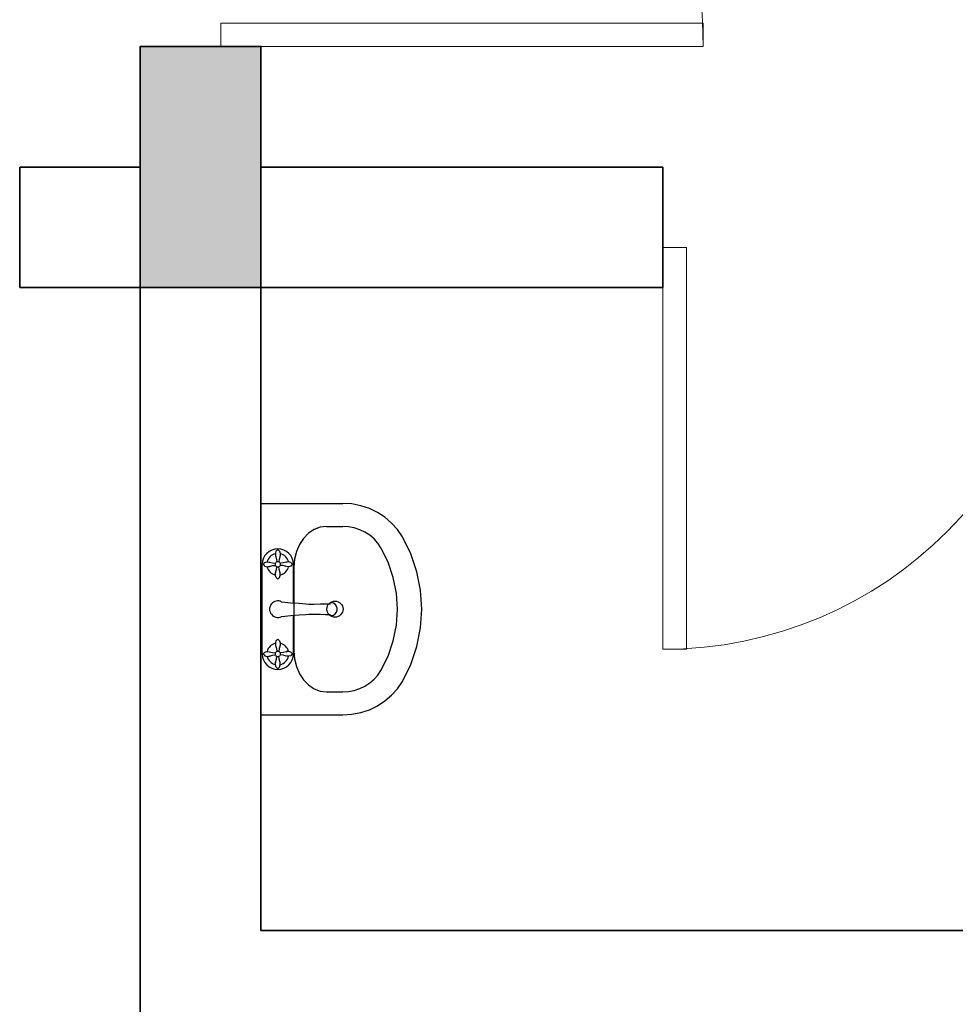
# Model space of a CAD drawing. Units: inches. Extents: x 3321 to 5237, y 11 to 1752.
# Tile 9 of 43: x 3654 to 3724, y 1372 to 1445. Entities that reach past the tile are written whole.
import ezdxf

# ---------------------------------------------------------------- set-up
doc = ezdxf.new("R2010")
doc.units = ezdxf.units.IN
for name, color, linetype, lineweight in [('A-ANNO-DIMS', 2, 'Continuous', 18), ('A-COLS', 1, 'Continuous', 35), ('A-DOOR', 4, 'Continuous', 18), ('A-WALL', 7, 'Continuous', 35), ('Сантехника', 7, 'Continuous', 18)]:
    doc.layers.add(name, color=color, linetype=linetype, lineweight=lineweight)
doc.layers.add('SANTEH', color=7, linetype='Continuous')
doc.styles.get("Standard").update_dxf_attribs({"font": 'arial.ttf'})
doc.dimstyles.new('ISO-25', dxfattribs={"dimtxt": 9, "dimasz": 2.5, "dimexe": 1.25, "dimexo": 0.625, "dimtad": 1, "dimdec": 1, "dimlunit": 3, "dimtxsty": 'Standard', "dimcen": 2.5, "dimclrd": 4, "dimclre": 4, "dimclrt": 256, "dimadec": 0, "dimazin": 0, "dimtfac": 1, "dimtdec": 1, "dimtmove": 0, "dimatfit": 3, "dimfxl": 1, "dimarcsym": 0})

# ---------------------------------------------------------------- blocks, each defined once
blk = doc.blocks.new('*U4')
for p, q in [((0, 0), (0, -6)), ((-36, 0), (-36, -6))]:
    blk.add_line(p, q)
blk.add_lwpolyline([(0, 0), (0, 36), (-1.75, 36), (-1.75, 0)], close=True)
blk.add_arc((0, 0), 36, 90, 180)
blk = doc.blocks.new('*U5')
for p, q in [((0, 0), (0, -6)), ((-30, 0), (-30, -6))]:
    blk.add_line(p, q)
blk.add_lwpolyline([(0, 0), (0, 30), (-1.75, 30), (-1.75, 0)], close=True)
blk.add_arc((0, 0), 30, 90, 180)
blk = doc.blocks.new('Basin 01_71')
at = {"layer": 'SANTEH'}
for p, q in [((0, 350), (0, 171.8)), ((460, 350), (0, 350)), ((130.2, 343.2), (128.5, 341.7)), ((130.2, 343.2), (128.5, 341.7)), ((130.2, 343.2), (128.5, 341.7)), ((130.2, 343.2), (128.5, 341.7)), ((130.2, 343.2), (128.5, 341.7)), ((130.2, 343.2), (128.5, 341.7)), ((132.5, 345.3), (130.2, 343.2)), ((132.5, 345.3), (130.2, 343.2)), ((132.5, 345.3), (130.2, 343.2)), ((132.5, 345.3), (130.2, 343.2)), ((132.5, 345.3), (130.2, 343.2)), ((132.5, 345.3), (130.2, 343.2)), ((132.5, 346.9), (327.5, 346.9)), ((132.5, 345.3), (134.7, 343.2)), ((132.5, 345.3), (134.7, 343.2)), ((132.5, 345.3), (134.7, 343.2)), ((132.5, 345.3), (134.7, 343.2)), ((132.5, 345.3), (134.7, 343.2)), ((132.5, 345.3), (134.7, 343.2)), ((134.7, 343.2), (136.4, 341.7)), ((134.7, 343.2), (136.4, 341.7)), ((134.7, 343.2), (136.4, 341.7)), ((134.7, 343.2), (136.4, 341.7)), ((134.7, 343.2), (136.4, 341.7)), ((134.7, 343.2), (136.4, 341.7)), ((325.2, 343.2), (323.5, 341.7)), ((325.2, 343.2), (323.5, 341.7)), ((325.2, 343.2), (323.5, 341.7)), ((325.2, 343.2), (323.5, 341.7)), ((325.2, 343.2), (323.5, 341.7)), ((325.2, 343.2), (323.5, 341.7)), ((327.5, 345.3), (325.2, 343.2)), ((327.5, 345.3), (325.2, 343.2)), ((327.5, 345.3), (325.2, 343.2)), ((327.5, 345.3), (325.2, 343.2)), ((327.5, 345.3), (325.2, 343.2)), ((327.5, 345.3), (325.2, 343.2)), ((327.5, 345.3), (329.7, 343.2)), ((327.5, 345.3), (329.7, 343.2)), ((327.5, 345.3), (329.7, 343.2)), ((327.5, 345.3), (329.7, 343.2)), ((327.5, 345.3), (329.7, 343.2)), ((327.5, 345.3), (329.7, 343.2)), ((329.7, 343.2), (331.4, 341.7)), ((329.7, 343.2), (331.4, 341.7)), ((329.7, 343.2), (331.4, 341.7)), ((329.7, 343.2), (331.4, 341.7)), ((329.7, 343.2), (331.4, 341.7)), ((329.7, 343.2), (331.4, 341.7)), ((460, 350), (460, 171.8)), ((128.5, 341.7), (127.2, 337.2)), ((128.5, 341.7), (127.2, 337.2)), ((128.5, 341.7), (127.2, 337.2)), ((128.5, 341.7), (127.2, 337.2)), ((128.5, 341.7), (127.2, 337.2)), ((128.5, 341.7), (127.2, 337.2)), ((127.2, 337.2), (127.5, 332.3)), ((127.2, 337.2), (127.5, 332.3)), ((127.2, 337.2), (127.5, 332.3)), ((127.2, 337.2), (127.5, 332.3)), ((127.2, 337.2), (127.5, 332.3)), ((127.2, 337.2), (127.5, 332.3)), ((127.5, 332.3), (128.4, 332)), ((127.5, 332.3), (128.4, 332)), ((127.5, 332.3), (128.4, 332)), ((127.5, 332.3), (128.4, 332)), ((127.5, 332.3), (128.4, 332)), ((127.5, 332.3), (128.4, 332)), ((128.4, 332), (127.6, 331.5)), ((128.4, 332), (127.6, 331.5)), ((128.4, 332), (127.6, 331.5)), ((128.4, 332), (127.6, 331.5)), ((128.4, 332), (127.6, 331.5)), ((128.4, 332), (127.6, 331.5)), ((127.6, 331.5), (129.6, 324.7)), ((127.6, 331.5), (129.6, 324.7)), ((127.6, 331.5), (129.6, 324.7)), ((127.6, 331.5), (129.6, 324.7)), ((127.6, 331.5), (129.6, 324.7)), ((127.6, 331.5), (129.6, 324.7)), ((129.6, 324.7), (130.2, 318.4)), ((129.6, 324.7), (130.2, 318.4)), ((129.6, 324.7), (130.2, 318.4)), ((129.6, 324.7), (130.2, 318.4)), ((129.6, 324.7), (130.2, 318.4)), ((129.6, 324.7), (130.2, 318.4)), ((135.4, 324.7), (134.8, 318.4)), ((135.4, 324.7), (134.8, 318.4)), ((135.4, 324.7), (134.8, 318.4)), ((135.4, 324.7), (134.8, 318.4)), ((135.4, 324.7), (134.8, 318.4)), ((135.4, 324.7), (134.8, 318.4)), ((137.4, 331.5), (135.4, 324.7)), ((137.4, 331.5), (135.4, 324.7)), ((137.4, 331.5), (135.4, 324.7)), ((137.4, 331.5), (135.4, 324.7)), ((137.4, 331.5), (135.4, 324.7)), ((137.4, 331.5), (135.4, 324.7)), ((136.4, 341.7), (137.7, 337.2)), ((136.4, 341.7), (137.7, 337.2)), ((136.4, 341.7), (137.7, 337.2)), ((136.4, 341.7), (137.7, 337.2)), ((136.4, 341.7), (137.7, 337.2)), ((136.4, 341.7), (137.7, 337.2)), ((137.4, 332.3), (136.6, 332)), ((137.4, 332.3), (136.6, 332)), ((137.4, 332.3), (136.6, 332)), ((137.4, 332.3), (136.6, 332)), ((137.4, 332.3), (136.6, 332)), ((137.4, 332.3), (136.6, 332)), ((136.6, 332), (137.4, 331.5)), ((136.6, 332), (137.4, 331.5)), ((136.6, 332), (137.4, 331.5)), ((136.6, 332), (137.4, 331.5)), ((136.6, 332), (137.4, 331.5)), ((136.6, 332), (137.4, 331.5)), ((137.7, 337.2), (137.4, 332.3)), ((137.7, 337.2), (137.4, 332.3)), ((137.7, 337.2), (137.4, 332.3)), ((137.7, 337.2), (137.4, 332.3)), ((137.7, 337.2), (137.4, 332.3)), ((137.7, 337.2), (137.4, 332.3)), ((323.5, 341.7), (322.2, 337.2)), ((323.5, 341.7), (322.2, 337.2)), ((323.5, 341.7), (322.2, 337.2)), ((323.5, 341.7), (322.2, 337.2)), ((323.5, 341.7), (322.2, 337.2)), ((323.5, 341.7), (322.2, 337.2)), ((322.2, 337.2), (322.5, 332.3)), ((322.2, 337.2), (322.5, 332.3)), ((322.2, 337.2), (322.5, 332.3)), ((322.2, 337.2), (322.5, 332.3)), ((322.2, 337.2), (322.5, 332.3)), ((322.2, 337.2), (322.5, 332.3)), ((322.5, 332.3), (323.4, 332)), ((322.5, 332.3), (323.4, 332)), ((322.5, 332.3), (323.4, 332)), ((322.5, 332.3), (323.4, 332)), ((322.5, 332.3), (323.4, 332)), ((322.5, 332.3), (323.4, 332)), ((323.4, 332), (322.6, 331.5)), ((323.4, 332), (322.6, 331.5)), ((323.4, 332), (322.6, 331.5)), ((323.4, 332), (322.6, 331.5)), ((323.4, 332), (322.6, 331.5)), ((323.4, 332), (322.6, 331.5)), ((322.6, 331.5), (324.6, 324.7)), ((322.6, 331.5), (324.6, 324.7)), ((322.6, 331.5), (324.6, 324.7)), ((322.6, 331.5), (324.6, 324.7)), ((322.6, 331.5), (324.6, 324.7)), ((322.6, 331.5), (324.6, 324.7)), ((324.6, 324.7), (325.2, 318.4)), ((324.6, 324.7), (325.2, 318.4)), ((324.6, 324.7), (325.2, 318.4)), ((324.6, 324.7), (325.2, 318.4)), ((324.6, 324.7), (325.2, 318.4)), ((324.6, 324.7), (325.2, 318.4)), ((330.4, 324.7), (329.8, 318.4)), ((330.4, 324.7), (329.8, 318.4)), ((330.4, 324.7), (329.8, 318.4)), ((330.4, 324.7), (329.8, 318.4)), ((330.4, 324.7), (329.8, 318.4)), ((330.4, 324.7), (329.8, 318.4)), ((332.4, 331.5), (330.4, 324.7)), ((332.4, 331.5), (330.4, 324.7)), ((332.4, 331.5), (330.4, 324.7)), ((332.4, 331.5), (330.4, 324.7)), ((332.4, 331.5), (330.4, 324.7)), ((332.4, 331.5), (330.4, 324.7)), ((331.4, 341.7), (332.7, 337.2)), ((331.4, 341.7), (332.7, 337.2)), ((331.4, 341.7), (332.7, 337.2)), ((331.4, 341.7), (332.7, 337.2)), ((331.4, 341.7), (332.7, 337.2)), ((331.4, 341.7), (332.7, 337.2)), ((332.4, 332.3), (331.6, 332)), ((332.4, 332.3), (331.6, 332)), ((332.4, 332.3), (331.6, 332)), ((332.4, 332.3), (331.6, 332)), ((332.4, 332.3), (331.6, 332)), ((332.4, 332.3), (331.6, 332)), ((331.6, 332), (332.4, 331.5)), ((331.6, 332), (332.4, 331.5)), ((331.6, 332), (332.4, 331.5)), ((331.6, 332), (332.4, 331.5)), ((331.6, 332), (332.4, 331.5)), ((331.6, 332), (332.4, 331.5)), ((332.7, 337.2), (332.4, 332.3)), ((332.7, 337.2), (332.4, 332.3)), ((332.7, 337.2), (332.4, 332.3)), ((332.7, 337.2), (332.4, 332.3)), ((332.7, 337.2), (332.4, 332.3)), ((332.7, 337.2), (332.4, 332.3)), ((100.4, 313.2), (102.5, 315.4)), ((100.4, 313.2), (102.5, 315.4)), ((100.4, 313.2), (102.5, 315.4)), ((100.4, 313.2), (102.5, 315.4)), ((100.4, 313.2), (102.5, 315.4)), ((100.4, 313.2), (102.5, 315.4)), ((100.4, 313.2), (102.5, 310.9)), ((100.4, 313.2), (102.5, 310.9)), ((100.4, 313.2), (102.5, 310.9)), ((100.4, 313.2), (102.5, 310.9)), ((100.4, 313.2), (102.5, 310.9)), ((100.4, 313.2), (102.5, 310.9)), ((102.5, 315.4), (104, 317.1)), ((102.5, 315.4), (104, 317.1)), ((102.5, 315.4), (104, 317.1)), ((102.5, 315.4), (104, 317.1)), ((102.5, 315.4), (104, 317.1)), ((102.5, 315.4), (104, 317.1)), ((102.5, 310.9), (104, 309.2)), ((102.5, 310.9), (104, 309.2)), ((102.5, 310.9), (104, 309.2)), ((102.5, 310.9), (104, 309.2)), ((102.5, 310.9), (104, 309.2)), ((102.5, 310.9), (104, 309.2)), ((104, 317.1), (108.5, 318.4)), ((104, 317.1), (108.5, 318.4)), ((104, 317.1), (108.5, 318.4)), ((104, 317.1), (108.5, 318.4)), ((104, 317.1), (108.5, 318.4)), ((104, 317.1), (108.5, 318.4)), ((104, 309.2), (108.5, 307.9)), ((104, 309.2), (108.5, 307.9)), ((104, 309.2), (108.5, 307.9)), ((104, 309.2), (108.5, 307.9)), ((104, 309.2), (108.5, 307.9)), ((104, 309.2), (108.5, 307.9)), ((108.5, 318.4), (113.4, 318.1)), ((108.5, 318.4), (113.4, 318.1)), ((108.5, 318.4), (113.4, 318.1)), ((108.5, 318.4), (113.4, 318.1)), ((108.5, 318.4), (113.4, 318.1)), ((108.5, 318.4), (113.4, 318.1)), ((108.5, 307.9), (113.4, 308.2)), ((108.5, 307.9), (113.4, 308.2)), ((108.5, 307.9), (113.4, 308.2)), ((108.5, 307.9), (113.4, 308.2)), ((108.5, 307.9), (113.4, 308.2)), ((108.5, 307.9), (113.4, 308.2)), ((113.4, 318.1), (113.7, 317.3)), ((113.4, 318.1), (113.7, 317.3)), ((113.4, 318.1), (113.7, 317.3)), ((113.4, 318.1), (113.7, 317.3)), ((113.4, 318.1), (113.7, 317.3)), ((113.4, 318.1), (113.7, 317.3)), ((113.4, 308.2), (113.7, 309.1)), ((113.4, 308.2), (113.7, 309.1)), ((113.4, 308.2), (113.7, 309.1)), ((113.4, 308.2), (113.7, 309.1)), ((113.4, 308.2), (113.7, 309.1)), ((113.4, 308.2), (113.7, 309.1)), ((113.7, 317.3), (114.2, 318.1)), ((113.7, 317.3), (114.2, 318.1)), ((113.7, 317.3), (114.2, 318.1)), ((113.7, 317.3), (114.2, 318.1)), ((113.7, 317.3), (114.2, 318.1)), ((113.7, 317.3), (114.2, 318.1)), ((113.7, 309.1), (114.2, 308.3)), ((113.7, 309.1), (114.2, 308.3)), ((113.7, 309.1), (114.2, 308.3)), ((113.7, 309.1), (114.2, 308.3)), ((113.7, 309.1), (114.2, 308.3)), ((113.7, 309.1), (114.2, 308.3)), ((114.2, 318.1), (121, 316.1)), ((114.2, 318.1), (121, 316.1)), ((114.2, 318.1), (121, 316.1)), ((114.2, 318.1), (121, 316.1)), ((114.2, 318.1), (121, 316.1)), ((114.2, 318.1), (121, 316.1)), ((114.2, 308.3), (121, 310.3)), ((114.2, 308.3), (121, 310.3)), ((114.2, 308.3), (121, 310.3)), ((114.2, 308.3), (121, 310.3)), ((114.2, 308.3), (121, 310.3)), ((114.2, 308.3), (121, 310.3)), ((121, 316.1), (127.3, 315.5)), ((121, 316.1), (127.3, 315.5)), ((121, 316.1), (127.3, 315.5)), ((121, 316.1), (127.3, 315.5)), ((121, 316.1), (127.3, 315.5)), ((121, 316.1), (127.3, 315.5)), ((121, 310.3), (127.3, 310.9)), ((121, 310.3), (127.3, 310.9)), ((121, 310.3), (127.3, 310.9)), ((121, 310.3), (127.3, 310.9)), ((121, 310.3), (127.3, 310.9)), ((121, 310.3), (127.3, 310.9)), ((127.1, 315.1), (126.8, 313.9)), ((127.1, 315.1), (126.8, 313.9)), ((127.1, 315.1), (126.8, 313.9)), ((127.1, 315.1), (126.8, 313.9)), ((127.1, 315.1), (126.8, 313.9)), ((127.1, 315.1), (126.8, 313.9)), ((126.8, 313.9), (126.8, 312.5)), ((126.8, 313.9), (126.8, 312.5)), ((126.8, 313.9), (126.8, 312.5)), ((126.8, 313.9), (126.8, 312.5)), ((126.8, 313.9), (126.8, 312.5)), ((126.8, 313.9), (126.8, 312.5)), ((126.8, 312.5), (127.1, 311.2)), ((126.8, 312.5), (127.1, 311.2)), ((126.8, 312.5), (127.1, 311.2)), ((126.8, 312.5), (127.1, 311.2)), ((126.8, 312.5), (127.1, 311.2)), ((126.8, 312.5), (127.1, 311.2)), ((127.7, 316.3), (127.1, 315.1)), ((127.7, 316.3), (127.1, 315.1)), ((127.7, 316.3), (127.1, 315.1)), ((127.7, 316.3), (127.1, 315.1)), ((127.7, 316.3), (127.1, 315.1)), ((127.7, 316.3), (127.1, 315.1)), ((127.1, 311.2), (127.7, 310.1)), ((127.1, 311.2), (127.7, 310.1)), ((127.1, 311.2), (127.7, 310.1)), ((127.1, 311.2), (127.7, 310.1)), ((127.1, 311.2), (127.7, 310.1)), ((127.1, 311.2), (127.7, 310.1)), ((127.6, 294.9), (129.6, 301.7)), ((127.6, 294.9), (129.6, 301.7)), ((127.6, 294.9), (129.6, 301.7)), ((127.6, 294.9), (129.6, 301.7)), ((127.6, 294.9), (129.6, 301.7)), ((127.6, 294.9), (129.6, 301.7)), ((128.6, 317.3), (127.7, 316.3)), ((128.6, 317.3), (127.7, 316.3)), ((128.6, 317.3), (127.7, 316.3)), ((128.6, 317.3), (127.7, 316.3)), ((128.6, 317.3), (127.7, 316.3)), ((128.6, 317.3), (127.7, 316.3)), ((127.7, 310.1), (128.6, 309.1)), ((127.7, 310.1), (128.6, 309.1)), ((127.7, 310.1), (128.6, 309.1)), ((127.7, 310.1), (128.6, 309.1)), ((127.7, 310.1), (128.6, 309.1)), ((127.7, 310.1), (128.6, 309.1)), ((129.7, 318.1), (128.6, 317.3)), ((129.7, 318.1), (128.6, 317.3)), ((129.7, 318.1), (128.6, 317.3)), ((129.7, 318.1), (128.6, 317.3)), ((129.7, 318.1), (128.6, 317.3)), ((129.7, 318.1), (128.6, 317.3)), ((128.6, 309.1), (129.7, 308.3)), ((128.6, 309.1), (129.7, 308.3)), ((128.6, 309.1), (129.7, 308.3)), ((128.6, 309.1), (129.7, 308.3)), ((128.6, 309.1), (129.7, 308.3)), ((128.6, 309.1), (129.7, 308.3)), ((129.6, 301.7), (130.2, 308)), ((129.6, 301.7), (130.2, 308)), ((129.6, 301.7), (130.2, 308)), ((129.6, 301.7), (130.2, 308)), ((129.6, 301.7), (130.2, 308)), ((129.6, 301.7), (130.2, 308)), ((130.9, 318.7), (129.7, 318.1)), ((130.9, 318.7), (129.7, 318.1)), ((130.9, 318.7), (129.7, 318.1)), ((130.9, 318.7), (129.7, 318.1)), ((130.9, 318.7), (129.7, 318.1)), ((130.9, 318.7), (129.7, 318.1)), ((129.7, 308.3), (130.9, 307.7)), ((129.7, 308.3), (130.9, 307.7)), ((129.7, 308.3), (130.9, 307.7)), ((129.7, 308.3), (130.9, 307.7)), ((129.7, 308.3), (130.9, 307.7)), ((129.7, 308.3), (130.9, 307.7)), ((132.2, 318.9), (130.9, 318.7)), ((132.2, 318.9), (130.9, 318.7)), ((132.2, 318.9), (130.9, 318.7)), ((132.2, 318.9), (130.9, 318.7)), ((132.2, 318.9), (130.9, 318.7)), ((132.2, 318.9), (130.9, 318.7)), ((130.9, 307.7), (132.2, 307.5)), ((130.9, 307.7), (132.2, 307.5)), ((130.9, 307.7), (132.2, 307.5)), ((130.9, 307.7), (132.2, 307.5)), ((130.9, 307.7), (132.2, 307.5)), ((130.9, 307.7), (132.2, 307.5)), ((133.5, 318.8), (132.2, 318.9)), ((133.5, 318.8), (132.2, 318.9)), ((133.5, 318.8), (132.2, 318.9)), ((133.5, 318.8), (132.2, 318.9)), ((133.5, 318.8), (132.2, 318.9)), ((133.5, 318.8), (132.2, 318.9)), ((132.2, 307.5), (133.5, 307.6)), ((132.2, 307.5), (133.5, 307.6)), ((132.2, 307.5), (133.5, 307.6)), ((132.2, 307.5), (133.5, 307.6)), ((132.2, 307.5), (133.5, 307.6)), ((132.2, 307.5), (133.5, 307.6)), ((134.8, 318.4), (133.5, 318.8)), ((134.8, 318.4), (133.5, 318.8)), ((134.8, 318.4), (133.5, 318.8)), ((134.8, 318.4), (133.5, 318.8)), ((134.8, 318.4), (133.5, 318.8)), ((134.8, 318.4), (133.5, 318.8)), ((133.5, 307.6), (134.8, 308)), ((133.5, 307.6), (134.8, 308)), ((133.5, 307.6), (134.8, 308)), ((133.5, 307.6), (134.8, 308)), ((133.5, 307.6), (134.8, 308)), ((133.5, 307.6), (134.8, 308)), ((135.9, 317.8), (134.8, 318.4)), ((135.9, 317.8), (134.8, 318.4)), ((135.9, 317.8), (134.8, 318.4)), ((135.9, 317.8), (134.8, 318.4)), ((135.9, 317.8), (134.8, 318.4)), ((135.9, 317.8), (134.8, 318.4)), ((134.8, 308), (135.9, 308.6)), ((134.8, 308), (135.9, 308.6)), ((134.8, 308), (135.9, 308.6)), ((134.8, 308), (135.9, 308.6)), ((134.8, 308), (135.9, 308.6)), ((134.8, 308), (135.9, 308.6)), ((135.4, 301.7), (134.8, 308)), ((135.4, 301.7), (134.8, 308)), ((135.4, 301.7), (134.8, 308)), ((135.4, 301.7), (134.8, 308)), ((135.4, 301.7), (134.8, 308)), ((135.4, 301.7), (134.8, 308)), ((137.4, 294.9), (135.4, 301.7)), ((137.4, 294.9), (135.4, 301.7)), ((137.4, 294.9), (135.4, 301.7)), ((137.4, 294.9), (135.4, 301.7)), ((137.4, 294.9), (135.4, 301.7)), ((137.4, 294.9), (135.4, 301.7)), ((136.9, 316.9), (135.9, 317.8)), ((136.9, 316.9), (135.9, 317.8)), ((136.9, 316.9), (135.9, 317.8)), ((136.9, 316.9), (135.9, 317.8)), ((136.9, 316.9), (135.9, 317.8)), ((136.9, 316.9), (135.9, 317.8)), ((135.9, 308.6), (136.9, 309.5)), ((135.9, 308.6), (136.9, 309.5)), ((135.9, 308.6), (136.9, 309.5)), ((135.9, 308.6), (136.9, 309.5)), ((135.9, 308.6), (136.9, 309.5)), ((135.9, 308.6), (136.9, 309.5)), ((137.6, 315.8), (136.9, 316.9)), ((137.6, 315.8), (136.9, 316.9)), ((137.6, 315.8), (136.9, 316.9)), ((137.6, 315.8), (136.9, 316.9)), ((137.6, 315.8), (136.9, 316.9)), ((137.6, 315.8), (136.9, 316.9)), ((136.9, 309.5), (137.6, 310.6)), ((136.9, 309.5), (137.6, 310.6)), ((136.9, 309.5), (137.6, 310.6)), ((136.9, 309.5), (137.6, 310.6)), ((136.9, 309.5), (137.6, 310.6)), ((136.9, 309.5), (137.6, 310.6)), ((138, 314.5), (137.6, 315.8)), ((138, 314.5), (137.6, 315.8)), ((138, 314.5), (137.6, 315.8)), ((138, 314.5), (137.6, 315.8)), ((138, 314.5), (137.6, 315.8)), ((138, 314.5), (137.6, 315.8)), ((137.6, 310.6), (138, 311.9)), ((137.6, 310.6), (138, 311.9)), ((137.6, 310.6), (138, 311.9)), ((137.6, 310.6), (138, 311.9)), ((137.6, 310.6), (138, 311.9)), ((137.6, 310.6), (138, 311.9)), ((144, 316.1), (137.7, 315.5)), ((144, 316.1), (137.7, 315.5)), ((144, 316.1), (137.7, 315.5)), ((144, 316.1), (137.7, 315.5)), ((144, 316.1), (137.7, 315.5)), ((144, 316.1), (137.7, 315.5)), ((144, 310.3), (137.7, 310.9)), ((144, 310.3), (137.7, 310.9)), ((144, 310.3), (137.7, 310.9)), ((144, 310.3), (137.7, 310.9)), ((144, 310.3), (137.7, 310.9)), ((144, 310.3), (137.7, 310.9)), ((138.2, 313.2), (138, 314.5)), ((138.2, 313.2), (138, 314.5)), ((138.2, 313.2), (138, 314.5)), ((138.2, 313.2), (138, 314.5)), ((138.2, 313.2), (138, 314.5)), ((138.2, 313.2), (138, 314.5)), ((138, 311.9), (138.2, 313.2)), ((138, 311.9), (138.2, 313.2)), ((138, 311.9), (138.2, 313.2)), ((138, 311.9), (138.2, 313.2)), ((138, 311.9), (138.2, 313.2)), ((138, 311.9), (138.2, 313.2)), ((150.8, 318.1), (144, 316.1)), ((150.8, 318.1), (144, 316.1)), ((150.8, 318.1), (144, 316.1)), ((150.8, 318.1), (144, 316.1)), ((150.8, 318.1), (144, 316.1)), ((150.8, 318.1), (144, 316.1)), ((150.8, 308.3), (144, 310.3)), ((150.8, 308.3), (144, 310.3)), ((150.8, 308.3), (144, 310.3)), ((150.8, 308.3), (144, 310.3)), ((150.8, 308.3), (144, 310.3)), ((150.8, 308.3), (144, 310.3)), ((151.3, 317.3), (150.8, 318.1)), ((151.3, 317.3), (150.8, 318.1)), ((151.3, 317.3), (150.8, 318.1)), ((151.3, 317.3), (150.8, 318.1)), ((151.3, 317.3), (150.8, 318.1)), ((151.3, 317.3), (150.8, 318.1)), ((151.3, 309.1), (150.8, 308.3)), ((151.3, 309.1), (150.8, 308.3)), ((151.3, 309.1), (150.8, 308.3)), ((151.3, 309.1), (150.8, 308.3)), ((151.3, 309.1), (150.8, 308.3)), ((151.3, 309.1), (150.8, 308.3)), ((151.6, 318.1), (151.3, 317.3)), ((151.6, 318.1), (151.3, 317.3)), ((151.6, 318.1), (151.3, 317.3)), ((151.6, 318.1), (151.3, 317.3)), ((151.6, 318.1), (151.3, 317.3)), ((151.6, 318.1), (151.3, 317.3)), ((151.6, 308.3), (151.3, 309.1)), ((151.6, 308.3), (151.3, 309.1)), ((151.6, 308.3), (151.3, 309.1)), ((151.6, 308.3), (151.3, 309.1)), ((151.6, 308.3), (151.3, 309.1)), ((151.6, 308.3), (151.3, 309.1)), ((156.5, 318.4), (151.6, 318.1)), ((156.5, 318.4), (151.6, 318.1)), ((156.5, 318.4), (151.6, 318.1)), ((156.5, 318.4), (151.6, 318.1)), ((156.5, 318.4), (151.6, 318.1)), ((156.5, 318.4), (151.6, 318.1)), ((156.5, 308), (151.6, 308.3)), ((156.5, 308), (151.6, 308.3)), ((156.5, 308), (151.6, 308.3)), ((156.5, 308), (151.6, 308.3)), ((156.5, 308), (151.6, 308.3)), ((156.5, 308), (151.6, 308.3)), ((161, 317.2), (156.5, 318.4)), ((161, 317.2), (156.5, 318.4)), ((161, 317.2), (156.5, 318.4)), ((161, 317.2), (156.5, 318.4)), ((161, 317.2), (156.5, 318.4)), ((161, 317.2), (156.5, 318.4)), ((161, 309.2), (156.5, 308)), ((161, 309.2), (156.5, 308)), ((161, 309.2), (156.5, 308)), ((161, 309.2), (156.5, 308)), ((161, 309.2), (156.5, 308)), ((161, 309.2), (156.5, 308)), ((162.5, 315.4), (161, 317.2)), ((162.5, 315.4), (161, 317.2)), ((162.5, 315.4), (161, 317.2)), ((162.5, 315.4), (161, 317.2)), ((162.5, 315.4), (161, 317.2)), ((162.5, 315.4), (161, 317.2)), ((162.5, 311), (161, 309.2)), ((162.5, 311), (161, 309.2)), ((162.5, 311), (161, 309.2)), ((162.5, 311), (161, 309.2)), ((162.5, 311), (161, 309.2)), ((162.5, 311), (161, 309.2)), ((164.6, 313.2), (162.5, 315.4)), ((164.6, 313.2), (162.5, 315.4)), ((164.6, 313.2), (162.5, 315.4)), ((164.6, 313.2), (162.5, 315.4)), ((164.6, 313.2), (162.5, 315.4)), ((164.6, 313.2), (162.5, 315.4)), ((164.6, 313.2), (162.5, 311)), ((164.6, 313.2), (162.5, 311)), ((164.6, 313.2), (162.5, 311)), ((164.6, 313.2), (162.5, 311)), ((164.6, 313.2), (162.5, 311)), ((164.6, 313.2), (162.5, 311)), ((213.9, 305.1), (215, 298)), ((246.1, 305.1), (245, 298)), ((295.4, 313.2), (297.5, 315.4)), ((295.4, 313.2), (297.5, 315.4)), ((295.4, 313.2), (297.5, 315.4)), ((295.4, 313.2), (297.5, 315.4)), ((295.4, 313.2), (297.5, 315.4)), ((295.4, 313.2), (297.5, 315.4)), ((295.4, 313.2), (297.5, 310.9)), ((295.4, 313.2), (297.5, 310.9)), ((295.4, 313.2), (297.5, 310.9)), ((295.4, 313.2), (297.5, 310.9)), ((295.4, 313.2), (297.5, 310.9)), ((295.4, 313.2), (297.5, 310.9)), ((297.5, 315.4), (299, 317.1)), ((297.5, 315.4), (299, 317.1)), ((297.5, 315.4), (299, 317.1)), ((297.5, 315.4), (299, 317.1)), ((297.5, 315.4), (299, 317.1)), ((297.5, 315.4), (299, 317.1)), ((297.5, 310.9), (299, 309.2)), ((297.5, 310.9), (299, 309.2)), ((297.5, 310.9), (299, 309.2)), ((297.5, 310.9), (299, 309.2)), ((297.5, 310.9), (299, 309.2)), ((297.5, 310.9), (299, 309.2)), ((299, 317.1), (303.5, 318.4)), ((299, 317.1), (303.5, 318.4)), ((299, 317.1), (303.5, 318.4)), ((299, 317.1), (303.5, 318.4)), ((299, 317.1), (303.5, 318.4)), ((299, 317.1), (303.5, 318.4)), ((299, 309.2), (303.5, 307.9)), ((299, 309.2), (303.5, 307.9)), ((299, 309.2), (303.5, 307.9)), ((299, 309.2), (303.5, 307.9)), ((299, 309.2), (303.5, 307.9)), ((299, 309.2), (303.5, 307.9)), ((303.5, 318.4), (308.4, 318.1)), ((303.5, 318.4), (308.4, 318.1)), ((303.5, 318.4), (308.4, 318.1)), ((303.5, 318.4), (308.4, 318.1)), ((303.5, 318.4), (308.4, 318.1)), ((303.5, 318.4), (308.4, 318.1)), ((303.5, 307.9), (308.4, 308.2)), ((303.5, 307.9), (308.4, 308.2)), ((303.5, 307.9), (308.4, 308.2)), ((303.5, 307.9), (308.4, 308.2)), ((303.5, 307.9), (308.4, 308.2)), ((303.5, 307.9), (308.4, 308.2)), ((308.4, 318.1), (308.7, 317.3)), ((308.4, 318.1), (308.7, 317.3)), ((308.4, 318.1), (308.7, 317.3)), ((308.4, 318.1), (308.7, 317.3)), ((308.4, 318.1), (308.7, 317.3)), ((308.4, 318.1), (308.7, 317.3)), ((308.4, 308.2), (308.7, 309.1)), ((308.4, 308.2), (308.7, 309.1)), ((308.4, 308.2), (308.7, 309.1)), ((308.4, 308.2), (308.7, 309.1)), ((308.4, 308.2), (308.7, 309.1)), ((308.4, 308.2), (308.7, 309.1)), ((308.7, 317.3), (309.2, 318.1)), ((308.7, 317.3), (309.2, 318.1)), ((308.7, 317.3), (309.2, 318.1)), ((308.7, 317.3), (309.2, 318.1)), ((308.7, 317.3), (309.2, 318.1)), ((308.7, 317.3), (309.2, 318.1)), ((308.7, 309.1), (309.2, 308.3)), ((308.7, 309.1), (309.2, 308.3)), ((308.7, 309.1), (309.2, 308.3)), ((308.7, 309.1), (309.2, 308.3)), ((308.7, 309.1), (309.2, 308.3)), ((308.7, 309.1), (309.2, 308.3)), ((309.2, 318.1), (316, 316.1)), ((309.2, 318.1), (316, 316.1)), ((309.2, 318.1), (316, 316.1)), ((309.2, 318.1), (316, 316.1)), ((309.2, 318.1), (316, 316.1)), ((309.2, 318.1), (316, 316.1)), ((309.2, 308.3), (316, 310.3)), ((309.2, 308.3), (316, 310.3)), ((309.2, 308.3), (316, 310.3)), ((309.2, 308.3), (316, 310.3)), ((309.2, 308.3), (316, 310.3)), ((309.2, 308.3), (316, 310.3)), ((316, 316.1), (322.3, 315.5)), ((316, 316.1), (322.3, 315.5)), ((316, 316.1), (322.3, 315.5)), ((316, 316.1), (322.3, 315.5)), ((316, 316.1), (322.3, 315.5)), ((316, 316.1), (322.3, 315.5)), ((316, 310.3), (322.3, 310.9)), ((316, 310.3), (322.3, 310.9)), ((316, 310.3), (322.3, 310.9)), ((316, 310.3), (322.3, 310.9)), ((316, 310.3), (322.3, 310.9)), ((316, 310.3), (322.3, 310.9)), ((322.1, 315.1), (321.8, 313.9)), ((322.1, 315.1), (321.8, 313.9)), ((322.1, 315.1), (321.8, 313.9)), ((322.1, 315.1), (321.8, 313.9)), ((322.1, 315.1), (321.8, 313.9)), ((322.1, 315.1), (321.8, 313.9)), ((321.8, 313.9), (321.8, 312.5)), ((321.8, 313.9), (321.8, 312.5)), ((321.8, 313.9), (321.8, 312.5)), ((321.8, 313.9), (321.8, 312.5)), ((321.8, 313.9), (321.8, 312.5)), ((321.8, 313.9), (321.8, 312.5)), ((321.8, 312.5), (322.1, 311.2)), ((321.8, 312.5), (322.1, 311.2)), ((321.8, 312.5), (322.1, 311.2)), ((321.8, 312.5), (322.1, 311.2)), ((321.8, 312.5), (322.1, 311.2)), ((321.8, 312.5), (322.1, 311.2)), ((322.7, 316.3), (322.1, 315.1)), ((322.7, 316.3), (322.1, 315.1)), ((322.7, 316.3), (322.1, 315.1)), ((322.7, 316.3), (322.1, 315.1)), ((322.7, 316.3), (322.1, 315.1)), ((322.7, 316.3), (322.1, 315.1)), ((322.1, 311.2), (322.7, 310.1)), ((322.1, 311.2), (322.7, 310.1)), ((322.1, 311.2), (322.7, 310.1)), ((322.1, 311.2), (322.7, 310.1)), ((322.1, 311.2), (322.7, 310.1)), ((322.1, 311.2), (322.7, 310.1)), ((322.6, 294.9), (324.6, 301.7)), ((322.6, 294.9), (324.6, 301.7)), ((322.6, 294.9), (324.6, 301.7)), ((322.6, 294.9), (324.6, 301.7)), ((322.6, 294.9), (324.6, 301.7)), ((322.6, 294.9), (324.6, 301.7)), ((323.6, 317.3), (322.7, 316.3)), ((323.6, 317.3), (322.7, 316.3)), ((323.6, 317.3), (322.7, 316.3)), ((323.6, 317.3), (322.7, 316.3)), ((323.6, 317.3), (322.7, 316.3)), ((323.6, 317.3), (322.7, 316.3)), ((322.7, 310.1), (323.6, 309.1)), ((322.7, 310.1), (323.6, 309.1)), ((322.7, 310.1), (323.6, 309.1)), ((322.7, 310.1), (323.6, 309.1)), ((322.7, 310.1), (323.6, 309.1)), ((322.7, 310.1), (323.6, 309.1)), ((324.7, 318.1), (323.6, 317.3)), ((324.7, 318.1), (323.6, 317.3)), ((324.7, 318.1), (323.6, 317.3)), ((324.7, 318.1), (323.6, 317.3)), ((324.7, 318.1), (323.6, 317.3)), ((324.7, 318.1), (323.6, 317.3)), ((323.6, 309.1), (324.7, 308.3)), ((323.6, 309.1), (324.7, 308.3)), ((323.6, 309.1), (324.7, 308.3)), ((323.6, 309.1), (324.7, 308.3)), ((323.6, 309.1), (324.7, 308.3)), ((323.6, 309.1), (324.7, 308.3)), ((324.6, 301.7), (325.2, 308)), ((324.6, 301.7), (325.2, 308)), ((324.6, 301.7), (325.2, 308)), ((324.6, 301.7), (325.2, 308)), ((324.6, 301.7), (325.2, 308)), ((324.6, 301.7), (325.2, 308)), ((325.9, 318.7), (324.7, 318.1)), ((325.9, 318.7), (324.7, 318.1)), ((325.9, 318.7), (324.7, 318.1)), ((325.9, 318.7), (324.7, 318.1)), ((325.9, 318.7), (324.7, 318.1)), ((325.9, 318.7), (324.7, 318.1)), ((324.7, 308.3), (325.9, 307.7)), ((324.7, 308.3), (325.9, 307.7)), ((324.7, 308.3), (325.9, 307.7)), ((324.7, 308.3), (325.9, 307.7)), ((324.7, 308.3), (325.9, 307.7)), ((324.7, 308.3), (325.9, 307.7)), ((327.2, 318.9), (325.9, 318.7)), ((327.2, 318.9), (325.9, 318.7)), ((327.2, 318.9), (325.9, 318.7)), ((327.2, 318.9), (325.9, 318.7)), ((327.2, 318.9), (325.9, 318.7)), ((327.2, 318.9), (325.9, 318.7)), ((325.9, 307.7), (327.2, 307.5)), ((325.9, 307.7), (327.2, 307.5)), ((325.9, 307.7), (327.2, 307.5)), ((325.9, 307.7), (327.2, 307.5)), ((325.9, 307.7), (327.2, 307.5)), ((325.9, 307.7), (327.2, 307.5)), ((328.5, 318.8), (327.2, 318.9)), ((328.5, 318.8), (327.2, 318.9)), ((328.5, 318.8), (327.2, 318.9)), ((328.5, 318.8), (327.2, 318.9)), ((328.5, 318.8), (327.2, 318.9)), ((328.5, 318.8), (327.2, 318.9)), ((327.2, 307.5), (328.5, 307.6)), ((327.2, 307.5), (328.5, 307.6)), ((327.2, 307.5), (328.5, 307.6)), ((327.2, 307.5), (328.5, 307.6)), ((327.2, 307.5), (328.5, 307.6)), ((327.2, 307.5), (328.5, 307.6)), ((329.8, 318.4), (328.5, 318.8)), ((329.8, 318.4), (328.5, 318.8)), ((329.8, 318.4), (328.5, 318.8)), ((329.8, 318.4), (328.5, 318.8)), ((329.8, 318.4), (328.5, 318.8)), ((329.8, 318.4), (328.5, 318.8)), ((328.5, 307.6), (329.8, 308)), ((328.5, 307.6), (329.8, 308)), ((328.5, 307.6), (329.8, 308)), ((328.5, 307.6), (329.8, 308)), ((328.5, 307.6), (329.8, 308)), ((328.5, 307.6), (329.8, 308)), ((330.9, 317.8), (329.8, 318.4)), ((330.9, 317.8), (329.8, 318.4)), ((330.9, 317.8), (329.8, 318.4)), ((330.9, 317.8), (329.8, 318.4)), ((330.9, 317.8), (329.8, 318.4)), ((330.9, 317.8), (329.8, 318.4)), ((329.8, 308), (330.9, 308.6)), ((329.8, 308), (330.9, 308.6)), ((329.8, 308), (330.9, 308.6)), ((329.8, 308), (330.9, 308.6)), ((329.8, 308), (330.9, 308.6)), ((329.8, 308), (330.9, 308.6)), ((330.4, 301.7), (329.8, 308)), ((330.4, 301.7), (329.8, 308)), ((330.4, 301.7), (329.8, 308)), ((330.4, 301.7), (329.8, 308)), ((330.4, 301.7), (329.8, 308)), ((330.4, 301.7), (329.8, 308)), ((332.4, 294.9), (330.4, 301.7)), ((332.4, 294.9), (330.4, 301.7)), ((332.4, 294.9), (330.4, 301.7)), ((332.4, 294.9), (330.4, 301.7)), ((332.4, 294.9), (330.4, 301.7)), ((332.4, 294.9), (330.4, 301.7)), ((331.9, 316.9), (330.9, 317.8)), ((331.9, 316.9), (330.9, 317.8)), ((331.9, 316.9), (330.9, 317.8)), ((331.9, 316.9), (330.9, 317.8)), ((331.9, 316.9), (330.9, 317.8)), ((331.9, 316.9), (330.9, 317.8)), ((330.9, 308.6), (331.9, 309.5)), ((330.9, 308.6), (331.9, 309.5)), ((330.9, 308.6), (331.9, 309.5)), ((330.9, 308.6), (331.9, 309.5)), ((330.9, 308.6), (331.9, 309.5)), ((330.9, 308.6), (331.9, 309.5)), ((332.6, 315.8), (331.9, 316.9)), ((332.6, 315.8), (331.9, 316.9)), ((332.6, 315.8), (331.9, 316.9)), ((332.6, 315.8), (331.9, 316.9)), ((332.6, 315.8), (331.9, 316.9)), ((332.6, 315.8), (331.9, 316.9)), ((331.9, 309.5), (332.6, 310.6)), ((331.9, 309.5), (332.6, 310.6)), ((331.9, 309.5), (332.6, 310.6)), ((331.9, 309.5), (332.6, 310.6)), ((331.9, 309.5), (332.6, 310.6)), ((331.9, 309.5), (332.6, 310.6)), ((333, 314.5), (332.6, 315.8)), ((333, 314.5), (332.6, 315.8)), ((333, 314.5), (332.6, 315.8)), ((333, 314.5), (332.6, 315.8)), ((333, 314.5), (332.6, 315.8)), ((333, 314.5), (332.6, 315.8)), ((332.6, 310.6), (333, 311.9)), ((332.6, 310.6), (333, 311.9)), ((332.6, 310.6), (333, 311.9)), ((332.6, 310.6), (333, 311.9)), ((332.6, 310.6), (333, 311.9)), ((332.6, 310.6), (333, 311.9)), ((339, 316.1), (332.7, 315.5)), ((339, 316.1), (332.7, 315.5)), ((339, 316.1), (332.7, 315.5)), ((339, 316.1), (332.7, 315.5)), ((339, 316.1), (332.7, 315.5)), ((339, 316.1), (332.7, 315.5)), ((339, 310.3), (332.7, 310.9)), ((339, 310.3), (332.7, 310.9)), ((339, 310.3), (332.7, 310.9)), ((339, 310.3), (332.7, 310.9)), ((339, 310.3), (332.7, 310.9)), ((339, 310.3), (332.7, 310.9)), ((333.2, 313.2), (333, 314.5)), ((333.2, 313.2), (333, 314.5)), ((333.2, 313.2), (333, 314.5)), ((333.2, 313.2), (333, 314.5)), ((333.2, 313.2), (333, 314.5)), ((333.2, 313.2), (333, 314.5)), ((333, 311.9), (333.2, 313.2)), ((333, 311.9), (333.2, 313.2)), ((333, 311.9), (333.2, 313.2)), ((333, 311.9), (333.2, 313.2)), ((333, 311.9), (333.2, 313.2)), ((333, 311.9), (333.2, 313.2)), ((345.8, 318.1), (339, 316.1)), ((345.8, 318.1), (339, 316.1)), ((345.8, 318.1), (339, 316.1)), ((345.8, 318.1), (339, 316.1)), ((345.8, 318.1), (339, 316.1)), ((345.8, 318.1), (339, 316.1)), ((345.8, 308.3), (339, 310.3)), ((345.8, 308.3), (339, 310.3)), ((345.8, 308.3), (339, 310.3)), ((345.8, 308.3), (339, 310.3)), ((345.8, 308.3), (339, 310.3)), ((345.8, 308.3), (339, 310.3)), ((346.3, 317.3), (345.8, 318.1)), ((346.3, 317.3), (345.8, 318.1)), ((346.3, 317.3), (345.8, 318.1)), ((346.3, 317.3), (345.8, 318.1)), ((346.3, 317.3), (345.8, 318.1)), ((346.3, 317.3), (345.8, 318.1)), ((346.3, 309.1), (345.8, 308.3)), ((346.3, 309.1), (345.8, 308.3)), ((346.3, 309.1), (345.8, 308.3)), ((346.3, 309.1), (345.8, 308.3)), ((346.3, 309.1), (345.8, 308.3)), ((346.3, 309.1), (345.8, 308.3)), ((346.6, 318.1), (346.3, 317.3)), ((346.6, 318.1), (346.3, 317.3)), ((346.6, 318.1), (346.3, 317.3)), ((346.6, 318.1), (346.3, 317.3)), ((346.6, 318.1), (346.3, 317.3)), ((346.6, 318.1), (346.3, 317.3)), ((346.6, 308.3), (346.3, 309.1)), ((346.6, 308.3), (346.3, 309.1)), ((346.6, 308.3), (346.3, 309.1)), ((346.6, 308.3), (346.3, 309.1)), ((346.6, 308.3), (346.3, 309.1)), ((346.6, 308.3), (346.3, 309.1)), ((351.5, 318.4), (346.6, 318.1)), ((351.5, 318.4), (346.6, 318.1)), ((351.5, 318.4), (346.6, 318.1)), ((351.5, 318.4), (346.6, 318.1)), ((351.5, 318.4), (346.6, 318.1)), ((351.5, 318.4), (346.6, 318.1)), ((351.5, 308), (346.6, 308.3)), ((351.5, 308), (346.6, 308.3)), ((351.5, 308), (346.6, 308.3)), ((351.5, 308), (346.6, 308.3)), ((351.5, 308), (346.6, 308.3)), ((351.5, 308), (346.6, 308.3)), ((356, 317.2), (351.5, 318.4)), ((356, 317.2), (351.5, 318.4)), ((356, 317.2), (351.5, 318.4)), ((356, 317.2), (351.5, 318.4)), ((356, 317.2), (351.5, 318.4)), ((356, 317.2), (351.5, 318.4)), ((356, 309.2), (351.5, 308)), ((356, 309.2), (351.5, 308)), ((356, 309.2), (351.5, 308)), ((356, 309.2), (351.5, 308)), ((356, 309.2), (351.5, 308)), ((356, 309.2), (351.5, 308)), ((357.5, 315.4), (356, 317.2)), ((357.5, 315.4), (356, 317.2)), ((357.5, 315.4), (356, 317.2)), ((357.5, 315.4), (356, 317.2)), ((357.5, 315.4), (356, 317.2)), ((357.5, 315.4), (356, 317.2)), ((357.5, 311), (356, 309.2)), ((357.5, 311), (356, 309.2)), ((357.5, 311), (356, 309.2)), ((357.5, 311), (356, 309.2)), ((357.5, 311), (356, 309.2)), ((357.5, 311), (356, 309.2)), ((359.6, 313.2), (357.5, 315.4)), ((359.6, 313.2), (357.5, 315.4)), ((359.6, 313.2), (357.5, 315.4)), ((359.6, 313.2), (357.5, 315.4)), ((359.6, 313.2), (357.5, 315.4)), ((359.6, 313.2), (357.5, 315.4)), ((359.6, 313.2), (357.5, 311)), ((359.6, 313.2), (357.5, 311)), ((359.6, 313.2), (357.5, 311)), ((359.6, 313.2), (357.5, 311)), ((359.6, 313.2), (357.5, 311)), ((359.6, 313.2), (357.5, 311)), ((127.3, 289.2), (127.6, 294.1)), ((127.3, 289.2), (127.6, 294.1)), ((127.3, 289.2), (127.6, 294.1)), ((127.3, 289.2), (127.6, 294.1)), ((127.3, 289.2), (127.6, 294.1)), ((127.3, 289.2), (127.6, 294.1)), ((128.6, 284.7), (127.3, 289.2)), ((128.6, 284.7), (127.3, 289.2)), ((128.6, 284.7), (127.3, 289.2)), ((128.6, 284.7), (127.3, 289.2)), ((128.6, 284.7), (127.3, 289.2)), ((128.6, 284.7), (127.3, 289.2)), ((128.4, 294.4), (127.6, 294.9)), ((128.4, 294.4), (127.6, 294.9)), ((128.4, 294.4), (127.6, 294.9)), ((128.4, 294.4), (127.6, 294.9)), ((128.4, 294.4), (127.6, 294.9)), ((128.4, 294.4), (127.6, 294.9)), ((127.6, 294.1), (128.4, 294.4)), ((127.6, 294.1), (128.4, 294.4)), ((127.6, 294.1), (128.4, 294.4)), ((127.6, 294.1), (128.4, 294.4)), ((127.6, 294.1), (128.4, 294.4)), ((127.6, 294.1), (128.4, 294.4)), ((130.3, 283.2), (128.6, 284.7)), ((130.3, 283.2), (128.6, 284.7)), ((130.3, 283.2), (128.6, 284.7)), ((130.3, 283.2), (128.6, 284.7)), ((130.3, 283.2), (128.6, 284.7)), ((130.3, 283.2), (128.6, 284.7)), ((132.5, 281.1), (130.3, 283.2)), ((132.5, 281.1), (130.3, 283.2)), ((132.5, 281.1), (130.3, 283.2)), ((132.5, 281.1), (130.3, 283.2)), ((132.5, 281.1), (130.3, 283.2)), ((132.5, 281.1), (130.3, 283.2)), ((132.5, 281.1), (134.8, 283.2)), ((132.5, 281.1), (134.8, 283.2)), ((132.5, 281.1), (134.8, 283.2)), ((132.5, 281.1), (134.8, 283.2)), ((132.5, 281.1), (134.8, 283.2)), ((132.5, 281.1), (134.8, 283.2)), ((132.5, 279.4), (216.5, 279.4)), ((134.8, 283.2), (136.5, 284.7)), ((134.8, 283.2), (136.5, 284.7)), ((134.8, 283.2), (136.5, 284.7)), ((134.8, 283.2), (136.5, 284.7)), ((134.8, 283.2), (136.5, 284.7)), ((134.8, 283.2), (136.5, 284.7)), ((136.5, 284.7), (137.8, 289.2)), ((136.5, 284.7), (137.8, 289.2)), ((136.5, 284.7), (137.8, 289.2)), ((136.5, 284.7), (137.8, 289.2)), ((136.5, 284.7), (137.8, 289.2)), ((136.5, 284.7), (137.8, 289.2)), ((136.6, 294.4), (137.4, 294.9)), ((136.6, 294.4), (137.4, 294.9)), ((136.6, 294.4), (137.4, 294.9)), ((136.6, 294.4), (137.4, 294.9)), ((136.6, 294.4), (137.4, 294.9)), ((136.6, 294.4), (137.4, 294.9)), ((137.5, 294.1), (136.6, 294.4)), ((137.5, 294.1), (136.6, 294.4)), ((137.5, 294.1), (136.6, 294.4)), ((137.5, 294.1), (136.6, 294.4)), ((137.5, 294.1), (136.6, 294.4)), ((137.5, 294.1), (136.6, 294.4)), ((137.8, 289.2), (137.5, 294.1)), ((137.8, 289.2), (137.5, 294.1)), ((137.8, 289.2), (137.5, 294.1)), ((137.8, 289.2), (137.5, 294.1)), ((137.8, 289.2), (137.5, 294.1)), ((137.8, 289.2), (137.5, 294.1)), ((215, 298), (216.2, 284.6)), ((216.2, 284.6), (217.3, 266.6)), ((243.8, 284.6), (242.7, 266.6)), ((243.5, 279.4), (327.5, 279.4)), ((245, 298), (243.8, 284.6)), ((322.3, 289.2), (322.6, 294.1)), ((322.3, 289.2), (322.6, 294.1)), ((322.3, 289.2), (322.6, 294.1)), ((322.3, 289.2), (322.6, 294.1)), ((322.3, 289.2), (322.6, 294.1)), ((322.3, 289.2), (322.6, 294.1)), ((323.6, 284.7), (322.3, 289.2)), ((323.6, 284.7), (322.3, 289.2)), ((323.6, 284.7), (322.3, 289.2)), ((323.6, 284.7), (322.3, 289.2)), ((323.6, 284.7), (322.3, 289.2)), ((323.6, 284.7), (322.3, 289.2)), ((323.4, 294.4), (322.6, 294.9)), ((323.4, 294.4), (322.6, 294.9)), ((323.4, 294.4), (322.6, 294.9)), ((323.4, 294.4), (322.6, 294.9)), ((323.4, 294.4), (322.6, 294.9)), ((323.4, 294.4), (322.6, 294.9)), ((322.6, 294.1), (323.4, 294.4)), ((322.6, 294.1), (323.4, 294.4)), ((322.6, 294.1), (323.4, 294.4)), ((322.6, 294.1), (323.4, 294.4)), ((322.6, 294.1), (323.4, 294.4)), ((322.6, 294.1), (323.4, 294.4)), ((325.3, 283.2), (323.6, 284.7)), ((325.3, 283.2), (323.6, 284.7)), ((325.3, 283.2), (323.6, 284.7)), ((325.3, 283.2), (323.6, 284.7)), ((325.3, 283.2), (323.6, 284.7)), ((325.3, 283.2), (323.6, 284.7)), ((327.5, 281.1), (325.3, 283.2)), ((327.5, 281.1), (325.3, 283.2)), ((327.5, 281.1), (325.3, 283.2)), ((327.5, 281.1), (325.3, 283.2)), ((327.5, 281.1), (325.3, 283.2)), ((327.5, 281.1), (325.3, 283.2)), ((327.5, 281.1), (329.8, 283.2)), ((327.5, 281.1), (329.8, 283.2)), ((327.5, 281.1), (329.8, 283.2)), ((327.5, 281.1), (329.8, 283.2)), ((327.5, 281.1), (329.8, 283.2)), ((327.5, 281.1), (329.8, 283.2)), ((329.8, 283.2), (331.5, 284.7)), ((329.8, 283.2), (331.5, 284.7)), ((329.8, 283.2), (331.5, 284.7)), ((329.8, 283.2), (331.5, 284.7)), ((329.8, 283.2), (331.5, 284.7)), ((329.8, 283.2), (331.5, 284.7)), ((331.5, 284.7), (332.8, 289.2)), ((331.5, 284.7), (332.8, 289.2)), ((331.5, 284.7), (332.8, 289.2)), ((331.5, 284.7), (332.8, 289.2)), ((331.5, 284.7), (332.8, 289.2)), ((331.5, 284.7), (332.8, 289.2)), ((331.6, 294.4), (332.4, 294.9)), ((331.6, 294.4), (332.4, 294.9)), ((331.6, 294.4), (332.4, 294.9)), ((331.6, 294.4), (332.4, 294.9)), ((331.6, 294.4), (332.4, 294.9)), ((331.6, 294.4), (332.4, 294.9)), ((332.5, 294.1), (331.6, 294.4)), ((332.5, 294.1), (331.6, 294.4)), ((332.5, 294.1), (331.6, 294.4)), ((332.5, 294.1), (331.6, 294.4)), ((332.5, 294.1), (331.6, 294.4)), ((332.5, 294.1), (331.6, 294.4)), ((332.8, 289.2), (332.5, 294.1)), ((332.8, 289.2), (332.5, 294.1)), ((332.8, 289.2), (332.5, 294.1)), ((332.8, 289.2), (332.5, 294.1)), ((332.8, 289.2), (332.5, 294.1)), ((332.8, 289.2), (332.5, 294.1)), ((138.9, 278.2), (138.9, 278.2)), ((321.1, 278.2), (138.9, 278.2)), ((217.3, 266.6), (218.3, 252.4)), ((242.7, 266.6), (241.7, 252.4)), ((218.3, 252.4), (219.3, 245.4)), ((219.3, 245.4), (219, 234.8)), ((241.7, 252.4), (240.7, 245.4)), ((240.7, 245.4), (241, 234.8)), ((218.8, 221.1), (218.6, 209.8)), ((219, 234.8), (218.8, 221.1)), ((241, 234.8), (241.2, 221.1)), ((241.2, 221.1), (241.4, 209.8)), ((50, 207.5), (50, 171.8)), ((217, 200.3), (216.2, 196.2)), ((216.2, 196.2), (217, 192.1)), ((217.1, 200.6), (217, 200.3)), ((218.5, 202.5), (217.1, 200.6)), ((218.6, 209.8), (218.4, 198.7)), ((241.4, 209.8), (241.6, 198.7)), ((242.9, 200.6), (241.5, 202.5)), ((242.9, 200.6), (243, 200.3)), ((243.8, 196.2), (243, 200.3)), ((243, 192.1), (243.8, 196.2)), ((410, 207.5), (410, 171.8)), ((217, 192.1), (217.1, 191.8)), ((217.1, 191.8), (219.5, 188.3)), ((219.5, 188.3), (223.2, 185.6)), ((223.2, 185.6), (227.6, 184.2)), ((227.6, 184.2), (227.7, 184.2)), ((227.7, 184.2), (232.3, 184.2)), ((232.4, 184.2), (232.3, 184.2)), ((232.4, 184.2), (236.8, 185.6)), ((236.8, 185.6), (240.5, 188.3)), ((240.5, 188.3), (242.9, 191.8)), ((243, 192.1), (242.9, 191.8))]:
    blk.add_line(p, q, dxfattribs=at)
for points in [[(138.9, 278.2), (121.6, 276.9), (104.9, 272.8), (89.5, 266.3), (76, 257.5), (65, 246.8), (56.8, 234.5), (51.7, 221.3), (50, 207.5)], [(410, 207.5), (408.3, 221.3), (403.2, 234.5), (395, 246.8), (384, 257.5), (370.5, 266.3), (355.1, 272.8), (338.4, 276.9), (321.1, 278.2)], [(0, 171.8), (1.2, 152.1), (5, 132.7), (11.1, 114.1), (19.5, 96.5), (30.1, 80.2), (42.7, 65.6), (56.9, 52.9), (72.7, 42.3)], [(50, 171.8), (50.8, 159.2), (53.2, 146.8), (57.1, 134.9), (62.5, 123.6), (69.3, 113.2), (77.3, 103.8), (86.4, 95.7), (96.5, 89)], [(363.5, 89), (373.6, 95.7), (382.7, 103.8), (390.7, 113.2), (397.5, 123.6), (402.9, 134.9), (406.8, 146.8), (409.2, 159.2), (410, 171.8)], [(387.3, 42.3), (403.1, 52.9), (417.3, 65.6), (429.9, 80.2), (440.5, 96.5), (448.9, 114.1), (455, 132.7), (458.8, 152.1), (460, 171.8)], [(96.5, 89), (128, 73.4), (161.1, 62.2), (195.3, 55.3), (230, 53), (264.7, 55.3), (298.9, 62.2), (332, 73.4), (363.5, 89)], [(72.7, 42.3), (109.8, 24), (148.8, 10.8), (189.1, 2.7), (230, 0), (270.9, 2.7), (311.2, 10.8), (350.2, 24), (387.3, 42.3)]]:
    blk.add_lwpolyline(points, dxfattribs=at)
blk.add_circle((230, 188.9), 17.5, dxfattribs=at)
for centre, radius, start, end in [((132.5, 313.2), 33.8, 90, 270), ((327.5, 313.2), 33.8, 270, 90), ((132.5, 313.2), 23.7, 102.6646, 167.4213), ((132.5, 313.2), 23.7, 12.6646, 77.4213), ((230, 313.2), 18, 333.1469, 206.8531), ((327.5, 313.2), 23.7, 102.5787, 167.3354), ((327.5, 313.2), 23.7, 12.5787, 77.3354), ((132.5, 313.2), 23.7, 192.6646, 257.4213), ((132.5, 313.2), 23.7, 282.6646, 347.4213), ((327.5, 313.2), 23.7, 192.5787, 257.3354), ((327.5, 313.2), 23.7, 282.5787, 347.3354)]:
    blk.add_arc(centre, radius, start, end, dxfattribs=at)
blk = doc.blocks.new('COL-9X18-IN')
h = blk.add_hatch(color=256)
h.dxf.hatch_style = 1
h.paths.add_polyline_path([(9, 18), (0, 18), (0, 0), (9, 0)])
blk.add_lwpolyline([(0, 0), (9, 0), (9, 18), (0, 18)], close=True)
blk = doc.blocks.new('*D192')
at = {"layer": 'A-ANNO-DIMS', "color": 4, "lineweight": -2, "transparency": 16777216}
for p, q in [((3704.375, 1473.484), (3704.375, 1457.036)), ((3791.689, 1473.484), (3791.689, 1457.036)), ((3706.875, 1458.286), (3789.189, 1458.286))]:
    blk.add_line(p, q, dxfattribs=at)
at = {"layer": 'A-ANNO-DIMS', "color": 4, "transparency": 16777216}
for points in [[(3706.875, 1458.702), (3706.875, 1457.869), (3704.375, 1458.286)], [(3789.189, 1458.702), (3789.189, 1457.869), (3791.689, 1458.286)]]:
    blk.add_solid(points, dxfattribs=at)
at = {"layer": 'Defpoints', "color": 0, "transparency": 16777216}
for p in [(3704.375, 1474.109), (3791.689, 1474.109), (3791.689, 1458.286)]:
    blk.add_point(p, dxfattribs=at)
at = {"layer": 'A-ANNO-DIMS', "transparency": 16777216, "insert": (3748.032, 1463.567), "char_height": 9, "attachment_point": 5}
blk.add_mtext('7\'-3 1/2" TYP.', dxfattribs=at)

msp = doc.modelspace()

# ---------------------------------------------------------------- linework, layer by layer
at = {"layer": 'A-WALL'}
for p, q in [((3662.689, 1443.339), (3671.689, 1443.339)), ((3662.689, 1443.339), (3662.689, 1434.339)), ((3671.689, 1443.339), (3671.689, 1434.339)), ((3653.689, 1434.339), (3662.689, 1434.339)), ((3653.689, 1434.339), (3653.689, 1425.339)), ((3671.689, 1434.339), (3701.689, 1434.339)), ((3701.689, 1425.339), (3701.689, 1434.339)), ((3653.689, 1425.339), (3662.689, 1425.339)), ((3662.689, 1425.339), (3662.689, 1307.339)), ((3671.689, 1425.339), (3701.689, 1425.339)), ((3671.689, 1425.339), (3671.689, 1377.339)), ((3671.689, 1377.339), (3791.689, 1377.339))]:
    msp.add_line(p, q, dxfattribs=at)

# ---------------------------------------------------------------- block references
at = {"layer": 'A-COLS'}
msp.add_blockref('COL-9X18-IN', (3662.689, 1425.339), dxfattribs=at)
at = {"layer": 'A-DOOR'}
for name, p, rotation in [('*U4', (3668.689, 1443.339), 270), ('*U5', (3701.689, 1428.339), 180)]:
    msp.add_blockref(name, p, dxfattribs=dict(at, rotation=rotation))
at = {"layer": 'Сантехника', "xscale": 0.0343047947041041, "yscale": 0.0343047947041041, "zscale": 0.0343047947041041, "rotation": 90.00000000000003}
msp.add_blockref('Basin 01_71', (3683.695, 1393.448), dxfattribs=at)

# ---------------------------------------------------------------- dimensions: what is measured, and where the dimension line sits
at = {"layer": 'A-ANNO-DIMS'}
dim = msp.add_linear_dim(base=(3791.689, 1458.286), p1=(3704.375, 1474.109), p2=(3791.689, 1474.109), text='<> TYP.', dimstyle='ISO-25', override={"dimdec": 1, "dimlfac": 1, "dimrnd": 0, "dimzin": 1, "dimdsep": 46, "dimlunit": 4, "dimfrac": 2}, dxfattribs=at)
dim.commit()
dim.dimension.update_dxf_attribs({"geometry": '*D192', "text_midpoint": (3748.032, 1463.567)})

doc.saveas('drawing.dxf')
